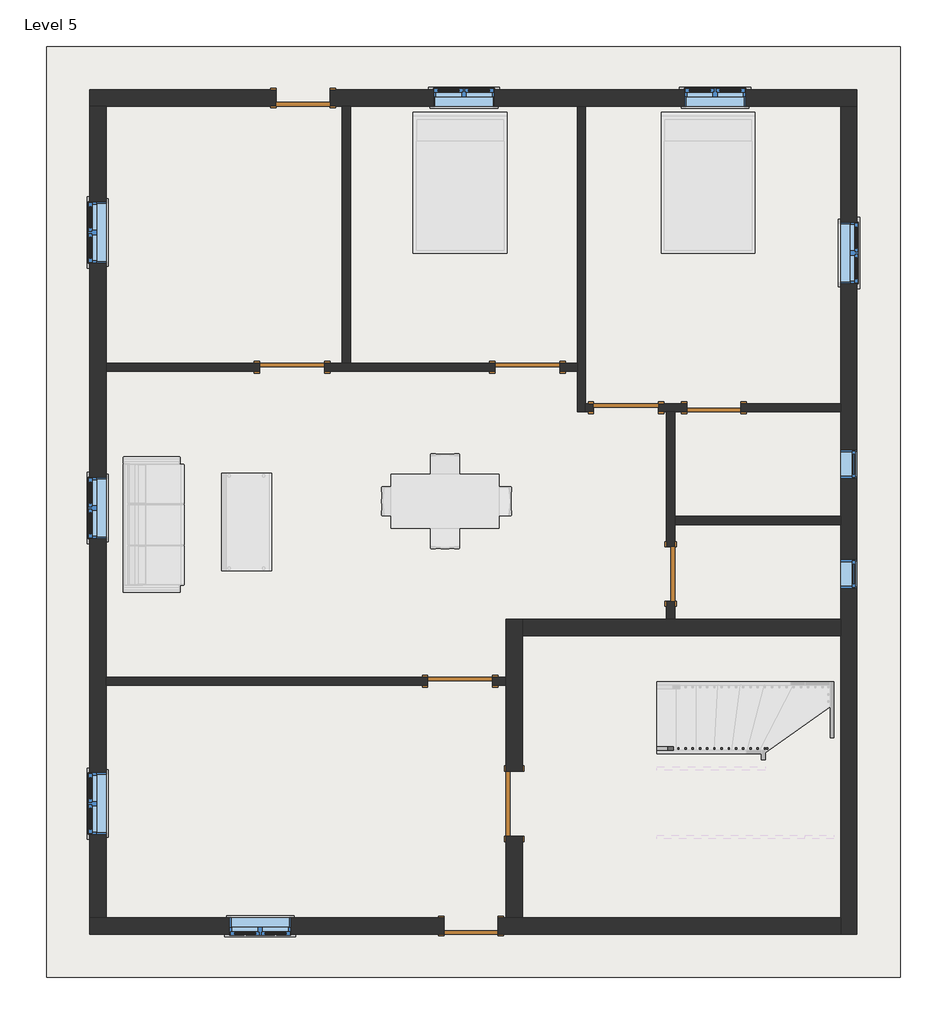
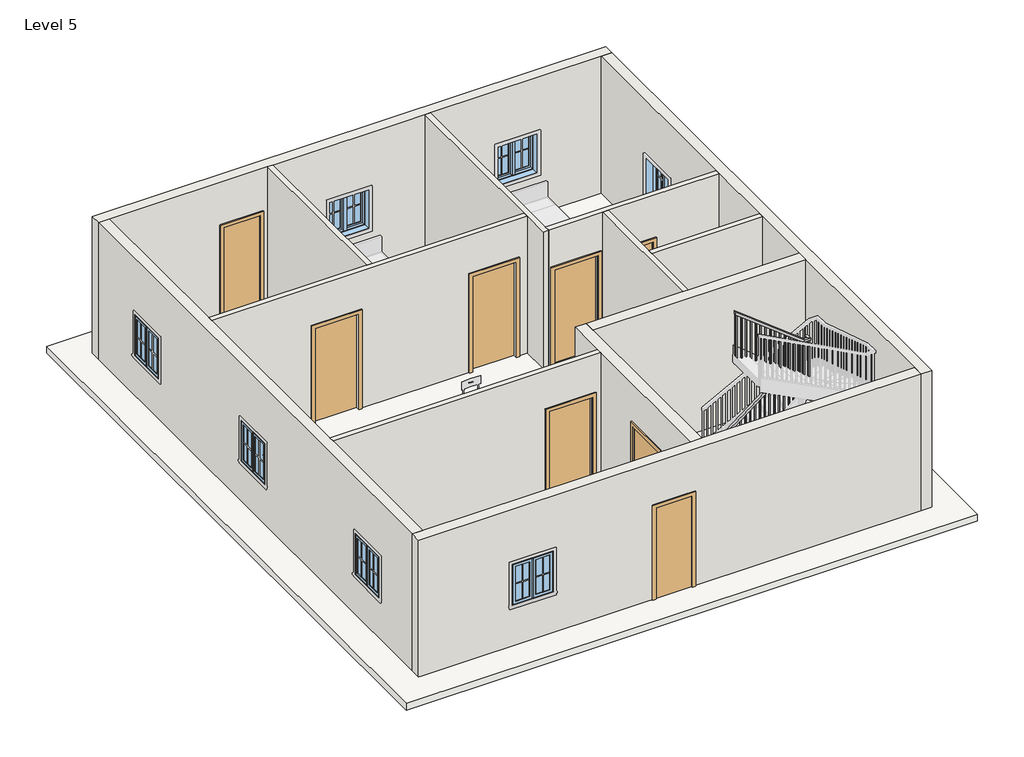
# One storey, part 1 of 2: 13 walls, 9 doors, 9 windows, 1 railing, 1 roof.
"""IFC4 building model written with IfcOpenShell, lengths in millimetres."""

from ifc_helpers import new_model, si_unit, frame, origin, place, context, project, spatial, polyline, outline, extrude, faceted_brep, transform, mapped, element, save
from components import door_85036156, door_d8f5dbb5, door_a1484949, door_e5f9f3c4, door_305aa2a5, door_0ca8825f, window_aa618e30, window_339605e1

model = new_model("IFC4")

# Units and contexts
model_context = context("Model", 3, world=origin())
ifc_project = project(units=[si_unit("LENGTHUNIT", "METRE", prefix="MILLI")], contexts=[model_context])

# Site, building, storey
site = spatial("IfcSite", under=ifc_project)
building = spatial("IfcBuilding", under=site)
storey = spatial("IfcBuildingStorey", under=building, Name="Level 5", Elevation=9601.2)

# Doors
placement = place(None, origin())
door_shape = door_85036156(model_context)
element("IfcDoor", 1, ObjectType="Single-Flush : 30\" x 80\"", at=placement, inside=storey, context=model_context, shape_type="MappedRepresentation", body=[
    mapped(door_shape, transform((-3639.3817864, 7024.9034997, 9601.2), x_axis=(1.0, 0.0, 0.0), y_axis=(0.0, 1.0, 0.0), z_axis=(0.0, 0.0, 1.0))),
])
door_2_shape = door_d8f5dbb5(model_context)
element("IfcDoor", 2, ObjectType="Single-Flush : 30\" x 80\"", at=placement, inside=storey, context=model_context, shape_type="MappedRepresentation", body=[
    mapped(door_2_shape, transform((2149.2782136, 2662.4534997, 9601.2), x_axis=(-1.0, 0.0, 0.0), y_axis=(0.0, -1.0, 0.0), z_axis=(0.0, 0.0, 1.0))),
])
element("IfcDoor", 3, ObjectType="Single-Flush : 30\" x 80\"", at=placement, inside=storey, context=model_context, shape_type="MappedRepresentation", body=[
    mapped(door_2_shape, transform((1539.6782136, 322.4784997, 9601.2), x_axis=(0.0, -1.0, 0.0), y_axis=(1.0, 0.0, 0.0), z_axis=(0.0, 0.0, 1.0))),
])
door_3_shape = door_a1484949(model_context)
element("IfcDoor", 4, ObjectType="Single-Flush : 30\" x 80\"", at=placement, inside=storey, context=model_context, shape_type="MappedRepresentation", body=[
    mapped(door_3_shape, transform((-1273.3717864, -4633.6965003, 9601.2), x_axis=(-1.0, 0.0, 0.0), y_axis=(0.0, -1.0, 0.0), z_axis=(0.0, 0.0, 1.0))),
])
door_4_shape = door_e5f9f3c4(model_context)
element("IfcDoor", 5, ObjectType="Single-Flush : 36\" x 84\"", at=placement, inside=storey, context=model_context, shape_type="MappedRepresentation", body=[
    mapped(door_4_shape, transform((-477.0817864, 3233.9534997, 9601.2), x_axis=(1.0, 0.0, 0.0), y_axis=(0.0, 1.0, 0.0), z_axis=(0.0, 0.0, 1.0))),
])
element("IfcDoor", 6, ObjectType="Single-Flush : 36\" x 84\"", at=placement, inside=storey, context=model_context, shape_type="MappedRepresentation", body=[
    mapped(door_4_shape, transform((-3791.7817864, 3233.9534997, 9601.2), x_axis=(1.0, 0.0, 0.0), y_axis=(0.0, 1.0, 0.0), z_axis=(0.0, 0.0, 1.0))),
])
element("IfcDoor", 7, ObjectType="Single-Flush : 36\" x 84\"", at=placement, inside=storey, context=model_context, shape_type="MappedRepresentation", body=[
    mapped(door_4_shape, transform((-1425.7717864, -1188.1865003, 9601.2), x_axis=(1.0, 0.0, 0.0), y_axis=(0.0, 1.0, 0.0), z_axis=(0.0, 0.0, 1.0))),
])
door_5_shape = door_305aa2a5(model_context)
element("IfcDoor", 8, ObjectType="Single-Flush : 36\" x 84\"", at=placement, inside=storey, context=model_context, shape_type="MappedRepresentation", body=[
    mapped(door_5_shape, transform((912.2982136, 2662.4534997, 9601.2), x_axis=(-1.0, 0.0, 0.0), y_axis=(0.0, -1.0, 0.0), z_axis=(0.0, 0.0, 1.0))),
])
door_6_shape = door_0ca8825f(model_context)
element("IfcDoor", 9, ObjectType="Single-Flush : 36\" x 84\"", at=placement, inside=storey, context=model_context, shape_type="MappedRepresentation", body=[
    mapped(door_6_shape, transform((-663.7717864, -2910.9415003, 9601.2), x_axis=(0.0, 1.0, 0.0), y_axis=(-1.0, 0.0, 0.0), z_axis=(0.0, 0.0, 1.0))),
])

# Railing
element("IfcRailing", 10, ObjectType="Handrail - Rectangular", at=placement, inside=storey, context=model_context, shape_type="SolidModel", body=[
    faceted_brep([(1342.8282136, -2108.9365003, 10684.9333333), (1342.8282136, -2108.9365003, 10620.6000346), (1342.8282136, -2159.7365003, 10620.6000346), (1342.8282136, -2159.7365003, 10684.9333333), (2794.3599055, -2108.9365003, 11812.8191036), (2845.1599055, -2108.9365003, 11787.9590024), (2845.1599055, -2159.7365003, 11787.9590024), (2794.3599055, -2159.7365003, 11812.8191036), (2794.3599055, -2108.9365003, 12015.8281882), (2845.1599055, -2108.9365003, 11965.0281882), (2845.1599055, -2159.7365003, 11965.0281882), (2794.3599055, -2159.7365003, 12015.8281882), (2921.3599055, -2108.9365003, 12015.8281882), (2921.3599055, -2108.9365003, 11965.0281882), (2870.5599055, -2159.7365003, 11965.0281882), (2870.5599055, -2159.7365003, 12015.8281882), (2921.3599055, -2235.9365003, 12015.8281882), (2921.3599055, -2265.0578342, 11965.0281882), (2870.5599055, -2265.0578342, 11965.0281882), (2870.5599055, -2235.9365003, 12015.8281882), (2921.3599055, -2362.9365003, 12232.7051451), (2921.3599055, -2413.7365003, 12218.9256424), (2870.5599055, -2413.7365003, 12218.9256424), (2870.5599055, -2362.9365003, 12232.7051451), (2921.3599055, -2362.9365003, 12435.7142297), (2921.3599055, -2413.7365003, 12384.9142297), (2870.5599055, -2413.7365003, 12384.9142297), (2870.5599055, -2362.9365003, 12435.7142297), (2921.3599055, -2489.9365003, 12435.7142297), (2921.3599055, -2489.9365003, 12384.9142297), (2870.5599055, -2439.1365003, 12384.9142297), (2870.5599055, -2439.1365003, 12435.7142297), (2794.3599055, -2489.9365003, 12435.7142297), (2776.9432376, -2489.9365003, 12384.9142297), (2776.9432376, -2439.1365003, 12384.9142297), (2794.3599055, -2439.1365003, 12435.7142297), (1342.8282136, -2489.9365003, 13563.6), (1342.8282136, -2439.1365003, 13563.6), (1342.8282136, -2439.1365003, 13499.2667013), (1342.8282136, -2489.9365003, 13499.2667013)], [[[0, 1, 2, 3]], [[1, 0, 4, 5]], [[2, 1, 5, 6]], [[3, 2, 6, 7]], [[0, 3, 7, 4]], [[5, 4, 8, 9]], [[6, 5, 9, 10]], [[7, 6, 10, 11]], [[4, 7, 11, 8]], [[9, 8, 12, 13]], [[10, 9, 13, 14]], [[11, 10, 14, 15]], [[8, 11, 15, 12]], [[13, 12, 16, 17]], [[14, 13, 17, 18]], [[15, 14, 18, 19]], [[12, 15, 19, 16]], [[17, 16, 20, 21]], [[18, 17, 21, 22]], [[19, 18, 22, 23]], [[16, 19, 23, 20]], [[21, 20, 24, 25]], [[22, 21, 25, 26]], [[23, 22, 26, 27]], [[20, 23, 27, 24]], [[25, 24, 28, 29]], [[26, 25, 29, 30]], [[27, 26, 30, 31]], [[24, 27, 31, 28]], [[29, 28, 32, 33]], [[30, 29, 33, 34]], [[31, 30, 34, 35]], [[28, 31, 35, 32]], [[36, 37, 38, 39]], [[33, 32, 36, 39]], [[34, 33, 39, 38]], [[35, 34, 38, 37]], [[32, 35, 37, 36]]]),
    extrude(outline(polyline([(13469.2292361, 1381.4849055), (13484.0316852, 1362.4349055), (12479.8666667, 1362.4349055), (12479.8666667, 1381.4849055), (13469.2292361, 1381.4849055)])), frame((0.0, -2474.0615003, 0.0), z_axis=(0.0, 1.0, 0.0), x_axis=(0.0, 0.0, 1.0)), (0.0, 0.0, 1.0), 19.05),
    extrude(outline(polyline([(13390.2828411, 1483.0849055), (13405.0852902, 1464.0349055), (12479.8666667, 1464.0349055), (12479.8666667, 1483.0849055), (13390.2828411, 1483.0849055)])), frame((0.0, -2474.0615003, 0.0), z_axis=(0.0, 1.0, 0.0), x_axis=(0.0, 0.0, 1.0)), (0.0, 0.0, 1.0), 19.05),
    extrude(outline(polyline([(13311.3364462, 1584.6849055), (13326.1388952, 1565.6349055), (12479.8666667, 1565.6349055), (12479.8666667, 1584.6849055), (13311.3364462, 1584.6849055)])), frame((0.0, -2474.0615003, 0.0), z_axis=(0.0, 1.0, 0.0), x_axis=(0.0, 0.0, 1.0)), (0.0, 0.0, 1.0), 19.05),
    extrude(outline(polyline([(13232.3900512, 1686.2849055), (13247.1925003, 1667.2349055), (12310.5333333, 1667.2349055), (12310.5333333, 1686.2849055), (13232.3900512, 1686.2849055)])), frame((0.0, -2474.0615003, 0.0), z_axis=(0.0, 1.0, 0.0), x_axis=(0.0, 0.0, 1.0)), (0.0, 0.0, 1.0), 19.05),
    extrude(outline(polyline([(13153.4436562, 1787.8849055), (13168.2461053, 1768.8349055), (12310.5333333, 1768.8349055), (12310.5333333, 1787.8849055), (13153.4436562, 1787.8849055)])), frame((0.0, -2474.0615003, 0.0), z_axis=(0.0, 1.0, 0.0), x_axis=(0.0, 0.0, 1.0)), (0.0, 0.0, 1.0), 19.05),
    extrude(outline(polyline([(13074.4972613, 1889.4849055), (13089.2997103, 1870.4349055), (12310.5333333, 1870.4349055), (12310.5333333, 1889.4849055), (13074.4972613, 1889.4849055)])), frame((0.0, -2474.0615003, 0.0), z_axis=(0.0, 1.0, 0.0), x_axis=(0.0, 0.0, 1.0)), (0.0, 0.0, 1.0), 19.05),
    extrude(outline(polyline([(12995.5508663, 1991.0849055), (13010.3533154, 1972.0349055), (12141.2, 1972.0349055), (12141.2, 1991.0849055), (12995.5508663, 1991.0849055)])), frame((0.0, -2474.0615003, 0.0), z_axis=(0.0, 1.0, 0.0), x_axis=(0.0, 0.0, 1.0)), (0.0, 0.0, 1.0), 19.05),
    extrude(outline(polyline([(12916.6044713, 2092.6849055), (12931.4069204, 2073.6349055), (12141.2, 2073.6349055), (12141.2, 2092.6849055), (12916.6044713, 2092.6849055)])), frame((0.0, -2474.0615003, 0.0), z_axis=(0.0, 1.0, 0.0), x_axis=(0.0, 0.0, 1.0)), (0.0, 0.0, 1.0), 19.05),
    extrude(outline(polyline([(12837.6580764, 2194.2849055), (12852.4605254, 2175.2349055), (11971.8666667, 2175.2349055), (11971.8666667, 2194.2849055), (12837.6580764, 2194.2849055)])), frame((0.0, -2474.0615003, 0.0), z_axis=(0.0, 1.0, 0.0), x_axis=(0.0, 0.0, 1.0)), (0.0, 0.0, 1.0), 19.05),
    extrude(outline(polyline([(12758.7116814, 2295.8849055), (12773.5141304, 2276.8349055), (11971.8666667, 2276.8349055), (11971.8666667, 2295.8849055), (12758.7116814, 2295.8849055)])), frame((0.0, -2474.0615003, 0.0), z_axis=(0.0, 1.0, 0.0), x_axis=(0.0, 0.0, 1.0)), (0.0, 0.0, 1.0), 19.05),
    extrude(outline(polyline([(12679.7652864, 2397.4849055), (12694.5677355, 2378.4349055), (11971.8666667, 2378.4349055), (11971.8666667, 2397.4849055), (12679.7652864, 2397.4849055)])), frame((0.0, -2474.0615003, 0.0), z_axis=(0.0, 1.0, 0.0), x_axis=(0.0, 0.0, 1.0)), (0.0, 0.0, 1.0), 19.05),
    extrude(outline(polyline([(12600.8188914, 2499.0849055), (12615.6213405, 2480.0349055), (11802.5333333, 2480.0349055), (11802.5333333, 2499.0849055), (12600.8188914, 2499.0849055)])), frame((0.0, -2474.0615003, 0.0), z_axis=(0.0, 1.0, 0.0), x_axis=(0.0, 0.0, 1.0)), (0.0, 0.0, 1.0), 19.05),
    extrude(outline(polyline([(12521.8724965, 2600.6849055), (12536.6749455, 2581.6349055), (11802.5333333, 2581.6349055), (11802.5333333, 2600.6849055), (12521.8724965, 2600.6849055)])), frame((0.0, -2474.0615003, 0.0), z_axis=(0.0, 1.0, 0.0), x_axis=(0.0, 0.0, 1.0)), (0.0, 0.0, 1.0), 19.05),
    extrude(outline(polyline([(12442.9261015, 2702.2849055), (12457.7285506, 2683.2349055), (11633.2, 2683.2349055), (11633.2, 2702.2849055), (12442.9261015, 2702.2849055)])), frame((0.0, -2474.0615003, 0.0), z_axis=(0.0, 1.0, 0.0), x_axis=(0.0, 0.0, 1.0)), (0.0, 0.0, 1.0), 19.05),
    extrude(outline(polyline([(12363.9797065, 2803.8849055), (12378.7821556, 2784.8349055), (11633.2, 2784.8349055), (11633.2, 2803.8849055), (12363.9797065, 2803.8849055)])), frame((0.0, -2474.0615003, 0.0), z_axis=(0.0, 1.0, 0.0), x_axis=(0.0, 0.0, 1.0)), (0.0, 0.0, 1.0), 19.05),
    extrude(outline(polyline([(2886.4349055, -2429.6115003), (2905.4849055, -2429.6115003), (2905.4849055, -2448.6615003), (2886.4349055, -2448.6615003), (2886.4349055, -2429.6115003)])), frame((0.0, 0.0, 11294.5333333), z_axis=(0.0, 0.0, 1.0), x_axis=(1.0, 0.0, 0.0)), (0.0, 0.0, 1.0), 1090.3808964),
    extrude(outline(polyline([(-2347.0615003, 12105.06524), (-2328.0115003, 12072.5336964), (-2328.0115003, 11125.2), (-2347.0615003, 11125.2), (-2347.0615003, 12105.06524)])), frame((2886.4349055, 0.0, 0.0), z_axis=(1.0, 0.0, 0.0), x_axis=(0.0, 1.0, 0.0)), (0.0, 0.0, 1.0), 19.05),
    extrude(outline(polyline([(-2245.4615003, 11931.5636744), (-2226.4115003, 11899.0321309), (-2226.4115003, 10955.8666667), (-2245.4615003, 10955.8666667), (-2245.4615003, 11931.5636744)])), frame((2886.4349055, 0.0, 0.0), z_axis=(1.0, 0.0, 0.0), x_axis=(0.0, 1.0, 0.0)), (0.0, 0.0, 1.0), 19.05),
    extrude(outline(polyline([(2857.3032136, -2143.8615003), (2857.3032136, -2124.8115003), (2876.3532136, -2124.8115003), (2876.3532136, -2143.8615003), (2857.3032136, -2143.8615003)])), frame((0.0, 0.0, 10786.5333333), z_axis=(0.0, 0.0, 1.0), x_axis=(1.0, 0.0, 0.0)), (0.0, 0.0, 1.0), 1178.4948549),
    extrude(outline(polyline([(11733.2507888, 2774.7532136), (11718.4483397, 2755.7032136), (10617.2, 2755.7032136), (10617.2, 2774.7532136), (11733.2507888, 2774.7532136)])), frame((0.0, -2143.8615003, 0.0), z_axis=(0.0, 1.0, 0.0), x_axis=(0.0, 0.0, 1.0)), (0.0, 0.0, 1.0), 19.05),
    extrude(outline(polyline([(11654.3043938, 2673.1532136), (11639.5019447, 2654.1032136), (10617.2, 2654.1032136), (10617.2, 2673.1532136), (11654.3043938, 2673.1532136)])), frame((0.0, -2143.8615003, 0.0), z_axis=(0.0, 1.0, 0.0), x_axis=(0.0, 0.0, 1.0)), (0.0, 0.0, 1.0), 19.05),
    extrude(outline(polyline([(11575.3579988, 2571.5532136), (11560.5555498, 2552.5032136), (10447.8666667, 2552.5032136), (10447.8666667, 2571.5532136), (11575.3579988, 2571.5532136)])), frame((0.0, -2143.8615003, 0.0), z_axis=(0.0, 1.0, 0.0), x_axis=(0.0, 0.0, 1.0)), (0.0, 0.0, 1.0), 19.05),
    extrude(outline(polyline([(11496.4116039, 2469.9532136), (11481.6091548, 2450.9032136), (10447.8666667, 2450.9032136), (10447.8666667, 2469.9532136), (11496.4116039, 2469.9532136)])), frame((0.0, -2143.8615003, 0.0), z_axis=(0.0, 1.0, 0.0), x_axis=(0.0, 0.0, 1.0)), (0.0, 0.0, 1.0), 19.05),
    extrude(outline(polyline([(11417.4652089, 2368.3532136), (11402.6627598, 2349.3032136), (10278.5333333, 2349.3032136), (10278.5333333, 2368.3532136), (11417.4652089, 2368.3532136)])), frame((0.0, -2143.8615003, 0.0), z_axis=(0.0, 1.0, 0.0), x_axis=(0.0, 0.0, 1.0)), (0.0, 0.0, 1.0), 19.05),
    extrude(outline(polyline([(11338.5188139, 2266.7532136), (11323.7163649, 2247.7032136), (10278.5333333, 2247.7032136), (10278.5333333, 2266.7532136), (11338.5188139, 2266.7532136)])), frame((0.0, -2143.8615003, 0.0), z_axis=(0.0, 1.0, 0.0), x_axis=(0.0, 0.0, 1.0)), (0.0, 0.0, 1.0), 19.05),
    extrude(outline(polyline([(11259.5724189, 2165.1532136), (11244.7699699, 2146.1032136), (10109.2, 2146.1032136), (10109.2, 2165.1532136), (11259.5724189, 2165.1532136)])), frame((0.0, -2143.8615003, 0.0), z_axis=(0.0, 1.0, 0.0), x_axis=(0.0, 0.0, 1.0)), (0.0, 0.0, 1.0), 19.05),
    extrude(outline(polyline([(11180.626024, 2063.5532136), (11165.8235749, 2044.5032136), (10109.2, 2044.5032136), (10109.2, 2063.5532136), (11180.626024, 2063.5532136)])), frame((0.0, -2143.8615003, 0.0), z_axis=(0.0, 1.0, 0.0), x_axis=(0.0, 0.0, 1.0)), (0.0, 0.0, 1.0), 19.05),
    extrude(outline(polyline([(11101.679629, 1961.9532136), (11086.8771799, 1942.9032136), (10109.2, 1942.9032136), (10109.2, 1961.9532136), (11101.679629, 1961.9532136)])), frame((0.0, -2143.8615003, 0.0), z_axis=(0.0, 1.0, 0.0), x_axis=(0.0, 0.0, 1.0)), (0.0, 0.0, 1.0), 19.05),
    extrude(outline(polyline([(11022.733234, 1860.3532136), (11007.930785, 1841.3032136), (9939.8666667, 1841.3032136), (9939.8666667, 1860.3532136), (11022.733234, 1860.3532136)])), frame((0.0, -2143.8615003, 0.0), z_axis=(0.0, 1.0, 0.0), x_axis=(0.0, 0.0, 1.0)), (0.0, 0.0, 1.0), 19.05),
    extrude(outline(polyline([(10943.7868391, 1758.7532136), (10928.98439, 1739.7032136), (9939.8666667, 1739.7032136), (9939.8666667, 1758.7532136), (10943.7868391, 1758.7532136)])), frame((0.0, -2143.8615003, 0.0), z_axis=(0.0, 1.0, 0.0), x_axis=(0.0, 0.0, 1.0)), (0.0, 0.0, 1.0), 19.05),
    extrude(outline(polyline([(10864.8404441, 1657.1532136), (10850.037995, 1638.1032136), (9939.8666667, 1638.1032136), (9939.8666667, 1657.1532136), (10864.8404441, 1657.1532136)])), frame((0.0, -2143.8615003, 0.0), z_axis=(0.0, 1.0, 0.0), x_axis=(0.0, 0.0, 1.0)), (0.0, 0.0, 1.0), 19.05),
    extrude(outline(polyline([(10785.8940491, 1555.5532136), (10771.0916001, 1536.5032136), (9770.5333333, 1536.5032136), (9770.5333333, 1555.5532136), (10785.8940491, 1555.5532136)])), frame((0.0, -2143.8615003, 0.0), z_axis=(0.0, 1.0, 0.0), x_axis=(0.0, 0.0, 1.0)), (0.0, 0.0, 1.0), 19.05),
    extrude(outline(polyline([(10706.9476541, 1453.9532136), (10692.1452051, 1434.9032136), (9770.5333333, 1434.9032136), (9770.5333333, 1453.9532136), (10706.9476541, 1453.9532136)])), frame((0.0, -2143.8615003, 0.0), z_axis=(0.0, 1.0, 0.0), x_axis=(0.0, 0.0, 1.0)), (0.0, 0.0, 1.0), 19.05),
    extrude(outline(polyline([(2886.4349055, -2455.0115003), (2905.4849055, -2455.0115003), (2905.4849055, -2474.0615003), (2886.4349055, -2474.0615003), (2886.4349055, -2455.0115003)])), frame((0.0, 0.0, 11463.8666667), z_axis=(0.0, 0.0, 1.0), x_axis=(1.0, 0.0, 0.0)), (0.0, 0.0, 1.0), 921.0475631),
    extrude(outline(polyline([(2886.4349055, -2143.8615003), (2886.4349055, -2124.8115003), (2905.4849055, -2124.8115003), (2905.4849055, -2143.8615003), (2886.4349055, -2143.8615003)])), frame((0.0, 0.0, 10786.5333333), z_axis=(0.0, 0.0, 1.0), x_axis=(1.0, 0.0, 0.0)), (0.0, 0.0, 1.0), 1178.4948549),
    extrude(outline(polyline([(13484.4642523, 1361.8782136), (13499.2667013, 1342.8282136), (12479.8666667, 1342.8282136), (12479.8666667, 1361.8782136), (13484.4642523, 1361.8782136)])), frame((0.0, -2474.0615003, 0.0), z_axis=(0.0, 1.0, 0.0), x_axis=(0.0, 0.0, 1.0)), (0.0, 0.0, 1.0), 19.05),
    extrude(outline(polyline([(10635.4024837, 1361.8782136), (10620.6000346, 1342.8282136), (9770.5333333, 1342.8282136), (9770.5333333, 1361.8782136), (10635.4024837, 1361.8782136)])), frame((0.0, -2143.8615003, 0.0), z_axis=(0.0, 1.0, 0.0), x_axis=(0.0, 0.0, 1.0)), (0.0, 0.0, 1.0), 19.05),
])

# Roof
element("IfcRoof", 11, ObjectType="Generic - 12\"", at=placement, inside=storey, context=model_context, shape_type="SweptSolid", body=[
    extrude(outline(polyline([(-7252.5317864, 7748.8034997), (4771.8282136, 7748.8034997), (4771.8282136, -5357.5965003), (-7252.5317864, -5357.5965003), (-7252.5317864, 7748.8034997)])), frame((0.0, 0.0, 9448.8), z_axis=(0.0, 0.0, 1.0), x_axis=(1.0, 0.0, 0.0)), (0.0, 0.0, 1.0), 152.4),
])

# Walls
element("IfcWall", 12, ObjectType="WALL4.5\"", at=placement, inside=storey, context=model_context, shape_type="Brep", body=[
    faceted_brep([(-3334.5817864, 3176.8034997, 11734.8), (-3334.5817864, 3176.8034997, 9601.2), (-934.2817864, 3176.8034997, 9601.2), (-934.2817864, 3176.8034997, 11734.8), (-19.8817864, 3176.8034997, 11734.8), (-19.8817864, 3176.8034997, 9601.2), (227.7682136, 3176.8034997, 9601.2), (227.7682136, 3176.8034997, 12649.2), (-6414.3317864, 3176.8034997, 12649.2), (-6414.3317864, 3176.8034997, 9601.2), (-4248.9817864, 3176.8034997, 9601.2), (-4248.9817864, 3176.8034997, 11734.8), (-934.2817864, 3291.1034997, 9601.2), (-2972.6317864, 3291.1034997, 9601.2), (-3086.9317864, 3291.1034997, 9601.2), (-3334.5817864, 3291.1034997, 9601.2), (-3334.5817864, 3291.1034997, 11734.8), (-4248.9817864, 3291.1034997, 11734.8), (-4248.9817864, 3291.1034997, 9601.2), (-6414.3317864, 3291.1034997, 9601.2), (-6414.3317864, 3291.1034997, 12649.2), (-3086.9317864, 3291.1034997, 12649.2), (-2972.6317864, 3291.1034997, 12649.2), (227.7682136, 3291.1034997, 12649.2), (227.7682136, 3291.1034997, 9601.2), (-19.8817864, 3291.1034997, 9601.2), (-19.8817864, 3291.1034997, 11734.8), (-934.2817864, 3291.1034997, 11734.8)], [[[0, 1, 2, 3, 4, 5, 6, 7, 8, 9, 10, 11]], [[12, 13, 14, 15, 16, 17, 18, 19, 20, 21, 22, 23, 24, 25, 26, 27]], [[6, 5, 25, 24]], [[10, 9, 19, 18]], [[2, 1, 15, 14, 13, 12]], [[9, 8, 20, 19]], [[7, 6, 24, 23]], [[26, 25, 5, 4]], [[27, 26, 4, 3]], [[12, 27, 3, 2]], [[16, 15, 1, 0]], [[17, 16, 0, 11]], [[18, 17, 11, 10]], [[8, 7, 23, 22, 21, 20]]]),
])
element("IfcWall", 13, ObjectType="WALL4.5\"", at=placement, inside=storey, context=model_context, shape_type="Brep", body=[
    faceted_brep([(227.7682136, 6910.6034997, 9601.2), (227.7682136, 3291.1034997, 9601.2), (227.7682136, 3176.8034997, 9601.2), (227.7682136, 2605.3034997, 9601.2), (227.7682136, 2605.3034997, 12649.2), (227.7682136, 3176.8034997, 12649.2), (227.7682136, 3291.1034997, 12649.2), (227.7682136, 6910.6034997, 12649.2), (342.0682136, 6910.6034997, 9601.2), (342.0682136, 6910.6034997, 12649.2), (342.0682136, 2719.6034997, 12649.2), (342.0682136, 2605.3034997, 12649.2), (342.0682136, 2605.3034997, 9601.2), (342.0682136, 2719.6034997, 9601.2)], [[[0, 1, 2, 3, 4, 5, 6, 7]], [[8, 9, 10, 11, 12, 13]], [[3, 2, 1, 0, 8, 13, 12]], [[0, 7, 9, 8]], [[4, 3, 12, 11]], [[7, 6, 5, 4, 11, 10, 9]]]),
])
element("IfcWall", 14, ObjectType="WALL4.5\"", at=placement, inside=storey, context=model_context, shape_type="Brep", body=[
    faceted_brep([(1369.4982136, 2605.3034997, 9601.2), (1482.5282136, 2605.3034997, 9601.2), (1596.8282136, 2605.3034997, 9601.2), (1768.2782136, 2605.3034997, 9601.2), (1768.2782136, 2605.3034997, 11633.2), (2530.2782136, 2605.3034997, 11633.2), (2530.2782136, 2605.3034997, 9601.2), (3933.6282136, 2605.3034997, 9601.2), (3933.6282136, 2605.3034997, 12649.2), (1596.8282136, 2605.3034997, 12649.2), (1482.5282136, 2605.3034997, 12649.2), (342.0682136, 2605.3034997, 12649.2), (342.0682136, 2605.3034997, 9601.2), (455.0982136, 2605.3034997, 9601.2), (455.0982136, 2605.3034997, 11734.8), (1369.4982136, 2605.3034997, 11734.8), (1768.2782136, 2719.6034997, 11633.2), (1768.2782136, 2719.6034997, 9601.2), (1369.4982136, 2719.6034997, 9601.2), (1369.4982136, 2719.6034997, 11734.8), (455.0982136, 2719.6034997, 11734.8), (455.0982136, 2719.6034997, 9601.2), (342.0682136, 2719.6034997, 9601.2), (342.0682136, 2719.6034997, 12649.2), (3933.6282136, 2719.6034997, 12649.2), (3933.6282136, 2719.6034997, 9601.2), (2530.2782136, 2719.6034997, 9601.2), (2530.2782136, 2719.6034997, 11633.2)], [[[0, 1, 2, 3, 4, 5, 6, 7, 8, 9, 10, 11, 12, 13, 14, 15]], [[16, 17, 18, 19, 20, 21, 22, 23, 24, 25, 26, 27]], [[22, 21, 13, 12]], [[26, 25, 7, 6]], [[18, 17, 3, 2, 1, 0]], [[12, 11, 23, 22]], [[8, 7, 25, 24]], [[14, 13, 21, 20]], [[15, 14, 20, 19]], [[0, 15, 19, 18]], [[4, 3, 17, 16]], [[5, 4, 16, 27]], [[6, 5, 27, 26]], [[11, 10, 9, 8, 24, 23]]]),
])
element("IfcWall", 15, ObjectType="WALL4.5\"", at=placement, inside=storey, context=model_context, shape_type="SweptSolid", body=[
    extrude(outline(polyline([(-3086.9317864, 3291.1034997), (-3086.9317864, 6910.6034997), (-2972.6317864, 6910.6034997), (-2972.6317864, 3291.1034997), (-3086.9317864, 3291.1034997)])), frame((0.0, 0.0, 9601.2), z_axis=(0.0, 0.0, 1.0), x_axis=(1.0, 0.0, 0.0)), (0.0, 0.0, 1.0), 3048.0),
])
element("IfcWall", 16, ObjectType="WALL4.5\"", at=placement, inside=storey, context=model_context, shape_type="Brep", body=[
    faceted_brep([(1482.5282136, -58.5215003, 11633.2), (1482.5282136, -58.5215003, 9601.2), (1482.5282136, -315.6965003, 9601.2), (1482.5282136, -315.6965003, 12649.2), (1482.5282136, 2605.3034997, 12649.2), (1482.5282136, 2605.3034997, 9601.2), (1482.5282136, 703.4784997, 9601.2), (1482.5282136, 703.4784997, 11633.2), (1596.8282136, -315.6965003, 9601.2), (1596.8282136, -58.5215003, 9601.2), (1596.8282136, -58.5215003, 11633.2), (1596.8282136, 703.4784997, 11633.2), (1596.8282136, 703.4784997, 9601.2), (1596.8282136, 1017.8034997, 9601.2), (1596.8282136, 1132.1034997, 9601.2), (1596.8282136, 2605.3034997, 9601.2), (1596.8282136, 2605.3034997, 12649.2), (1596.8282136, 1132.1034997, 12649.2), (1596.8282136, 1017.8034997, 12649.2), (1596.8282136, -315.6965003, 12649.2)], [[[0, 1, 2, 3, 4, 5, 6, 7]], [[8, 9, 10, 11, 12, 13, 14, 15, 16, 17, 18, 19]], [[6, 5, 15, 14, 13, 12]], [[2, 1, 9, 8]], [[5, 4, 16, 15]], [[3, 2, 8, 19]], [[10, 9, 1, 0]], [[11, 10, 0, 7]], [[12, 11, 7, 6]], [[4, 3, 19, 18, 17, 16]]]),
])
element("IfcWall", 17, ObjectType="WALL4.5\"", at=placement, inside=storey, context=model_context, shape_type="SweptSolid", body=[
    extrude(outline(polyline([(3933.6282136, 1017.8034997), (1596.8282136, 1017.8034997), (1596.8282136, 1132.1034997), (3933.6282136, 1132.1034997), (3933.6282136, 1017.8034997)])), frame((0.0, 0.0, 9601.2), z_axis=(0.0, 0.0, 1.0), x_axis=(1.0, 0.0, 0.0)), (0.0, 0.0, 1.0), 3048.0),
])
element("IfcWall", 18, ObjectType="WALL4.5\"", at=placement, inside=storey, context=model_context, shape_type="SweptSolid", body=[
    extrude(outline(polyline([(11734.8, -968.5717864), (9601.2, -968.5717864), (9601.2, -778.0717864), (12649.2, -778.0717864), (12649.2, -6414.3317864), (9601.2, -6414.3317864), (9601.2, -1882.9717864), (11734.8, -1882.9717864), (11734.8, -968.5717864)])), frame((0.0, -1245.3365003, 0.0), z_axis=(0.0, 1.0, 0.0), x_axis=(0.0, 0.0, 1.0)), (0.0, 0.0, 1.0), 114.3),
])
element("IfcWall", 19, ObjectType="WALL9\"", at=placement, inside=storey, context=model_context, shape_type="Brep", body=[
    faceted_brep([(-3258.3817864, 6910.6034997, 11633.2), (-3258.3817864, 6910.6034997, 9601.2), (-3086.9317864, 6910.6034997, 9601.2), (-2972.6317864, 6910.6034997, 9601.2), (227.7682136, 6910.6034997, 9601.2), (342.0682136, 6910.6034997, 9601.2), (3933.6282136, 6910.6034997, 9601.2), (4162.2282136, 6910.6034997, 9601.2), (4162.2282136, 6910.6034997, 12649.2), (3933.6282136, 6910.6034997, 12649.2), (342.0682136, 6910.6034997, 12649.2), (227.7682136, 6910.6034997, 12649.2), (-2972.6317864, 6910.6034997, 12649.2), (-3086.9317864, 6910.6034997, 12649.2), (-6414.3317864, 6910.6034997, 12649.2), (-6642.9317864, 6910.6034997, 12649.2), (-6642.9317864, 6910.6034997, 9601.2), (-6414.3317864, 6910.6034997, 9601.2), (-4020.3817864, 6910.6034997, 9601.2), (-4020.3817864, 6910.6034997, 11633.2), (-940.6317864, 6910.6034997, 11430.0), (-940.6317864, 6910.6034997, 10515.6), (-1804.2317864, 6910.6034997, 10515.6), (-1804.2317864, 6910.6034997, 11430.0), (2598.2232136, 6910.6034997, 11430.0), (2598.2232136, 6910.6034997, 10515.6), (1734.6232136, 6910.6034997, 10515.6), (1734.6232136, 6910.6034997, 11430.0), (4162.2282136, 7139.2034997, 9601.2), (-3258.3817864, 7139.2034997, 9601.2), (-3258.3817864, 7139.2034997, 11633.2), (-4020.3817864, 7139.2034997, 11633.2), (-4020.3817864, 7139.2034997, 9601.2), (-6642.9317864, 7139.2034997, 9601.2), (-6642.9317864, 7139.2034997, 12649.2), (4162.2282136, 7139.2034997, 12649.2), (-940.6317864, 7139.2034997, 11430.0), (-1804.2317864, 7139.2034997, 11430.0), (-1804.2317864, 7139.2034997, 10515.6), (-940.6317864, 7139.2034997, 10515.6), (2598.2232136, 7139.2034997, 11430.0), (1734.6232136, 7139.2034997, 11430.0), (1734.6232136, 7139.2034997, 10515.6), (2598.2232136, 7139.2034997, 10515.6)], [[[0, 1, 2, 3, 4, 5, 6, 7, 8, 9, 10, 11, 12, 13, 14, 15, 16, 17, 18, 19], [20, 21, 22, 23], [24, 25, 26, 27]], [[28, 29, 30, 31, 32, 33, 34, 35], [36, 37, 38, 39], [40, 41, 42, 43]], [[18, 17, 16, 33, 32]], [[7, 6, 5, 4, 3, 2, 1, 29, 28]], [[8, 7, 28, 35]], [[16, 15, 34, 33]], [[30, 29, 1, 0]], [[31, 30, 0, 19]], [[32, 31, 19, 18]], [[21, 20, 36, 39]], [[22, 21, 39, 38]], [[23, 22, 38, 37]], [[20, 23, 37, 36]], [[25, 24, 40, 43]], [[26, 25, 43, 42]], [[27, 26, 42, 41]], [[24, 27, 41, 40]], [[15, 14, 13, 12, 11, 10, 9, 8, 35, 34]]]),
])
element("IfcWall", 20, ObjectType="WALL9\"", at=placement, inside=storey, context=model_context, shape_type="Brep", body=[
    faceted_brep([(3933.6282136, 6910.6034997, 9601.2), (3933.6282136, 2719.6034997, 9601.2), (3933.6282136, 2605.3034997, 9601.2), (3933.6282136, 1132.1034997, 9601.2), (3933.6282136, 1017.8034997, 9601.2), (3933.6282136, -315.6965003, 9601.2), (3933.6282136, -544.2965003, 9601.2), (3933.6282136, -4519.3965003, 9601.2), (3933.6282136, -4747.9965003, 9601.2), (3933.6282136, -4747.9965003, 12649.2), (3933.6282136, -4519.3965003, 12649.2), (3933.6282136, -544.2965003, 12649.2), (3933.6282136, -315.6965003, 12649.2), (3933.6282136, 1017.8034997, 12649.2), (3933.6282136, 1132.1034997, 12649.2), (3933.6282136, 2605.3034997, 12649.2), (3933.6282136, 2719.6034997, 12649.2), (3933.6282136, 6910.6034997, 12649.2), (3933.6282136, 1665.5034997, 11125.2), (3933.6282136, 1665.5034997, 10515.6), (3933.6282136, 2071.9034997, 10515.6), (3933.6282136, 2071.9034997, 11125.2), (3933.6282136, 119.2784997, 11125.2), (3933.6282136, 119.2784997, 10515.6), (3933.6282136, 525.6784997, 10515.6), (3933.6282136, 525.6784997, 11125.2), (3933.6282136, 4411.8784997, 11430.0), (3933.6282136, 4411.8784997, 10515.6), (3933.6282136, 5275.4784997, 10515.6), (3933.6282136, 5275.4784997, 11430.0), (4162.2282136, 6910.6034997, 9601.2), (4162.2282136, 6910.6034997, 12649.2), (4162.2282136, -4747.9965003, 12649.2), (4162.2282136, -4747.9965003, 9601.2), (4162.2282136, 1665.5034997, 11125.2), (4162.2282136, 2071.9034997, 11125.2), (4162.2282136, 2071.9034997, 10515.6), (4162.2282136, 1665.5034997, 10515.6), (4162.2282136, 119.2784997, 11125.2), (4162.2282136, 525.6784997, 11125.2), (4162.2282136, 525.6784997, 10515.6), (4162.2282136, 119.2784997, 10515.6), (4162.2282136, 4411.8784997, 11430.0), (4162.2282136, 5275.4784997, 11430.0), (4162.2282136, 5275.4784997, 10515.6), (4162.2282136, 4411.8784997, 10515.6)], [[[0, 1, 2, 3, 4, 5, 6, 7, 8, 9, 10, 11, 12, 13, 14, 15, 16, 17], [18, 19, 20, 21], [22, 23, 24, 25], [26, 27, 28, 29]], [[30, 31, 32, 33], [34, 35, 36, 37], [38, 39, 40, 41], [42, 43, 44, 45]], [[8, 7, 6, 5, 4, 3, 2, 1, 0, 30, 33]], [[0, 17, 31, 30]], [[9, 8, 33, 32]], [[19, 18, 34, 37]], [[20, 19, 37, 36]], [[21, 20, 36, 35]], [[18, 21, 35, 34]], [[23, 22, 38, 41]], [[24, 23, 41, 40]], [[25, 24, 40, 39]], [[22, 25, 39, 38]], [[27, 26, 42, 45]], [[28, 27, 45, 44]], [[29, 28, 44, 43]], [[26, 29, 43, 42]], [[17, 16, 15, 14, 13, 12, 11, 10, 9, 32, 31]]]),
])
element("IfcWall", 21, ObjectType="WALL9\"", at=placement, inside=storey, context=model_context, shape_type="Brep", body=[
    faceted_brep([(-1654.3717864, -4519.3965003, 11633.2), (-1654.3717864, -4519.3965003, 9601.2), (-6414.3317864, -4519.3965003, 9601.2), (-6642.9317864, -4519.3965003, 9601.2), (-6642.9317864, -4519.3965003, 12649.2), (-6414.3317864, -4519.3965003, 12649.2), (-778.0717864, -4519.3965003, 12649.2), (-549.4717864, -4519.3965003, 12649.2), (3933.6282136, -4519.3965003, 12649.2), (3933.6282136, -4519.3965003, 9601.2), (-549.4717864, -4519.3965003, 9601.2), (-778.0717864, -4519.3965003, 9601.2), (-892.3717864, -4519.3965003, 9601.2), (-892.3717864, -4519.3965003, 11633.2), (-4674.4317864, -4519.3965003, 11430.0), (-4674.4317864, -4519.3965003, 10515.6), (-3810.8317864, -4519.3965003, 10515.6), (-3810.8317864, -4519.3965003, 11430.0), (-6642.9317864, -4747.9965003, 9601.2), (-1654.3717864, -4747.9965003, 9601.2), (-1654.3717864, -4747.9965003, 11633.2), (-892.3717864, -4747.9965003, 11633.2), (-892.3717864, -4747.9965003, 9601.2), (3933.6282136, -4747.9965003, 9601.2), (3933.6282136, -4747.9965003, 12649.2), (-6642.9317864, -4747.9965003, 12649.2), (-4674.4317864, -4747.9965003, 11430.0), (-3810.8317864, -4747.9965003, 11430.0), (-3810.8317864, -4747.9965003, 10515.6), (-4674.4317864, -4747.9965003, 10515.6)], [[[0, 1, 2, 3, 4, 5, 6, 7, 8, 9, 10, 11, 12, 13], [14, 15, 16, 17]], [[18, 19, 20, 21, 22, 23, 24, 25], [26, 27, 28, 29]], [[3, 2, 1, 19, 18]], [[12, 11, 10, 9, 23, 22]], [[9, 8, 24, 23]], [[4, 3, 18, 25]], [[15, 14, 26, 29]], [[16, 15, 29, 28]], [[17, 16, 28, 27]], [[14, 17, 27, 26]], [[8, 7, 6, 5, 4, 25, 24]], [[20, 19, 1, 0]], [[21, 20, 0, 13]], [[22, 21, 13, 12]]]),
])
element("IfcWall", 22, ObjectType="WALL9\"", at=placement, inside=storey, context=model_context, shape_type="Brep", body=[
    faceted_brep([(-6414.3317864, -4519.3965003, 9601.2), (-6414.3317864, -1245.3365003, 9601.2), (-6414.3317864, -1131.0365003, 9601.2), (-6414.3317864, 3176.8034997, 9601.2), (-6414.3317864, 3291.1034997, 9601.2), (-6414.3317864, 6910.6034997, 9601.2), (-6414.3317864, 6910.6034997, 12649.2), (-6414.3317864, 3291.1034997, 12649.2), (-6414.3317864, 3176.8034997, 12649.2), (-6414.3317864, -1131.0365003, 12649.2), (-6414.3317864, -1245.3365003, 12649.2), (-6414.3317864, -4519.3965003, 12649.2), (-6414.3317864, 5561.2284997, 11430.0), (-6414.3317864, 5561.2284997, 10515.6), (-6414.3317864, 4697.6284997, 10515.6), (-6414.3317864, 4697.6284997, 11430.0), (-6414.3317864, 1684.5534997, 11430.0), (-6414.3317864, 1684.5534997, 10515.6), (-6414.3317864, 820.9534997, 10515.6), (-6414.3317864, 820.9534997, 11430.0), (-6414.3317864, -2479.1415003, 11430.0), (-6414.3317864, -2479.1415003, 10515.6), (-6414.3317864, -3342.7415003, 10515.6), (-6414.3317864, -3342.7415003, 11430.0), (-6642.9317864, -4519.3965003, 9601.2), (-6642.9317864, -4519.3965003, 12649.2), (-6642.9317864, 6910.6034997, 12649.2), (-6642.9317864, 6910.6034997, 9601.2), (-6642.9317864, 5561.2284997, 11430.0), (-6642.9317864, 4697.6284997, 11430.0), (-6642.9317864, 4697.6284997, 10515.6), (-6642.9317864, 5561.2284997, 10515.6), (-6642.9317864, 1684.5534997, 11430.0), (-6642.9317864, 820.9534997, 11430.0), (-6642.9317864, 820.9534997, 10515.6), (-6642.9317864, 1684.5534997, 10515.6), (-6642.9317864, -2479.1415003, 11430.0), (-6642.9317864, -3342.7415003, 11430.0), (-6642.9317864, -3342.7415003, 10515.6), (-6642.9317864, -2479.1415003, 10515.6)], [[[0, 1, 2, 3, 4, 5, 6, 7, 8, 9, 10, 11], [12, 13, 14, 15], [16, 17, 18, 19], [20, 21, 22, 23]], [[24, 25, 26, 27], [28, 29, 30, 31], [32, 33, 34, 35], [36, 37, 38, 39]], [[5, 4, 3, 2, 1, 0, 24, 27]], [[0, 11, 25, 24]], [[6, 5, 27, 26]], [[13, 12, 28, 31]], [[14, 13, 31, 30]], [[15, 14, 30, 29]], [[12, 15, 29, 28]], [[17, 16, 32, 35]], [[18, 17, 35, 34]], [[19, 18, 34, 33]], [[16, 19, 33, 32]], [[21, 20, 36, 39]], [[22, 21, 39, 38]], [[23, 22, 38, 37]], [[20, 23, 37, 36]], [[11, 10, 9, 8, 7, 6, 26, 25]]]),
])
element("IfcWall", 23, ObjectType="WALL9\"", at=placement, inside=storey, context=model_context, shape_type="Brep", body=[
    faceted_brep([(-549.4717864, -2453.7415003, 11734.8), (-549.4717864, -2453.7415003, 9601.2), (-549.4717864, -544.2965003, 9601.2), (-549.4717864, -315.6965003, 9601.2), (-549.4717864, -315.6965003, 12649.2), (-549.4717864, -544.2965003, 12649.2), (-549.4717864, -4519.3965003, 12649.2), (-549.4717864, -4519.3965003, 9601.2), (-549.4717864, -3368.1415003, 9601.2), (-549.4717864, -3368.1415003, 11734.8), (-778.0717864, -315.6965003, 9601.2), (-778.0717864, -1131.0365003, 9601.2), (-778.0717864, -1245.3365003, 9601.2), (-778.0717864, -2453.7415003, 9601.2), (-778.0717864, -2453.7415003, 11734.8), (-778.0717864, -3368.1415003, 11734.8), (-778.0717864, -3368.1415003, 9601.2), (-778.0717864, -4519.3965003, 9601.2), (-778.0717864, -4519.3965003, 12649.2), (-778.0717864, -1245.3365003, 12649.2), (-778.0717864, -1131.0365003, 12649.2), (-778.0717864, -315.6965003, 12649.2)], [[[0, 1, 2, 3, 4, 5, 6, 7, 8, 9]], [[10, 11, 12, 13, 14, 15, 16, 17, 18, 19, 20, 21]], [[8, 7, 17, 16]], [[3, 2, 1, 13, 12, 11, 10]], [[7, 6, 18, 17]], [[4, 3, 10, 21]], [[14, 13, 1, 0]], [[15, 14, 0, 9]], [[16, 15, 9, 8]], [[6, 5, 4, 21, 20, 19, 18]]]),
])
element("IfcWall", 24, ObjectType="WALL9\"", at=placement, inside=storey, context=model_context, shape_type="Brep", body=[
    faceted_brep([(-549.4717864, -544.2965003, 9601.2), (3933.6282136, -544.2965003, 9601.2), (3933.6282136, -544.2965003, 12649.2), (-549.4717864, -544.2965003, 12649.2), (-549.4717864, -315.6965003, 9601.2), (-549.4717864, -315.6965003, 12649.2), (1482.5282136, -315.6965003, 12649.2), (1596.8282136, -315.6965003, 12649.2), (3933.6282136, -315.6965003, 12649.2), (3933.6282136, -315.6965003, 9601.2), (1596.8282136, -315.6965003, 9601.2), (1482.5282136, -315.6965003, 9601.2)], [[[0, 1, 2, 3]], [[4, 5, 6, 7, 8, 9, 10, 11]], [[1, 0, 4, 11, 10, 9]], [[0, 3, 5, 4]], [[2, 1, 9, 8]], [[3, 2, 8, 7, 6, 5]]]),
])

# Windows
window_shape = window_aa618e30(model_context)
element("IfcWindow", 25, ObjectType="Fixed : 16\" x 24\"", at=placement, inside=storey, context=model_context, shape_type="MappedRepresentation", body=[
    mapped(window_shape, transform((4047.9282136, 1830.6034997, 9601.2), x_axis=(0.0, -1.0, 0.0), y_axis=(1.0, 0.0, 0.0), z_axis=(0.0, 0.0, 1.0))),
])
element("IfcWindow", 26, ObjectType="Fixed : 16\" x 24\"", at=placement, inside=storey, context=model_context, shape_type="MappedRepresentation", body=[
    mapped(window_shape, transform((4047.9282136, 284.3784997, 9601.2), x_axis=(0.0, -1.0, 0.0), y_axis=(1.0, 0.0, 0.0), z_axis=(0.0, 0.0, 1.0))),
])
window_2_shape = window_339605e1(model_context)
element("IfcWindow", 27, ObjectType="Window-Casement-Double : 34\" x 36\"", at=placement, inside=storey, context=model_context, shape_type="MappedRepresentation", body=[
    mapped(window_2_shape, transform((-1372.4317864, 7024.9034997, 9601.2), x_axis=(1.0, 0.0, 0.0), y_axis=(0.0, 1.0, 0.0), z_axis=(0.0, 0.0, 1.0))),
])
element("IfcWindow", 28, ObjectType="Window-Casement-Double : 34\" x 36\"", at=placement, inside=storey, context=model_context, shape_type="MappedRepresentation", body=[
    mapped(window_2_shape, transform((2166.4232136, 7024.9034997, 9601.2), x_axis=(1.0, 0.0, 0.0), y_axis=(0.0, 1.0, 0.0), z_axis=(0.0, 0.0, 1.0))),
])
element("IfcWindow", 29, ObjectType="Window-Casement-Double : 34\" x 36\"", at=placement, inside=storey, context=model_context, shape_type="MappedRepresentation", body=[
    mapped(window_2_shape, transform((-6528.6317864, 5129.4284997, 9601.2), x_axis=(0.0, 1.0, 0.0), y_axis=(-1.0, 0.0, 0.0), z_axis=(0.0, 0.0, 1.0))),
])
element("IfcWindow", 30, ObjectType="Window-Casement-Double : 34\" x 36\"", at=placement, inside=storey, context=model_context, shape_type="MappedRepresentation", body=[
    mapped(window_2_shape, transform((-6528.6317864, 1252.7534997, 9601.2), x_axis=(0.0, 1.0, 0.0), y_axis=(-1.0, 0.0, 0.0), z_axis=(0.0, 0.0, 1.0))),
])
element("IfcWindow", 31, ObjectType="Window-Casement-Double : 34\" x 36\"", at=placement, inside=storey, context=model_context, shape_type="MappedRepresentation", body=[
    mapped(window_2_shape, transform((4047.9282136, 4843.6784997, 9601.2), x_axis=(0.0, -1.0, 0.0), y_axis=(1.0, 0.0, 0.0), z_axis=(0.0, 0.0, 1.0))),
])
element("IfcWindow", 32, ObjectType="Window-Casement-Double : 34\" x 36\"", at=placement, inside=storey, context=model_context, shape_type="MappedRepresentation", body=[
    mapped(window_2_shape, transform((-6528.6317864, -2910.9415003, 9601.2), x_axis=(0.0, 1.0, 0.0), y_axis=(-1.0, 0.0, 0.0), z_axis=(0.0, 0.0, 1.0))),
])
element("IfcWindow", 33, ObjectType="Window-Casement-Double : 34\" x 36\"", at=placement, inside=storey, context=model_context, shape_type="MappedRepresentation", body=[
    mapped(window_2_shape, transform((-4242.6317864, -4633.6965003, 9601.2), x_axis=(-1.0, 0.0, 0.0), y_axis=(0.0, -1.0, 0.0), z_axis=(0.0, 0.0, 1.0))),
])

save(model, "model.ifc")

# Revit data of these elements
# Type "Single-Flush : 30\" x 80\""
#   Type Mark = "5"
#   Construction Type Id = "MDOOR"
#   Assembly Code = "C1020"
#   Analytic Construction = "Metal"
#   Thickness = 0' - 2"
#   Heat Transfer Coefficient (U) = 0.651978 BTU/(h·ft²·°F)
#   Height = 6' - 8"
#   Trim Projection Ext = 0' - 1"
#   Trim Projection Int = 0' - 1"
#   Trim Width = 0' - 3"
#   Width = 2' - 6"
#   Define Thermal Properties by = 1
#   Define Thermal Properties by = 1
#   Door Material = Door - Panel
#   Frame Material = Door - Frame
#   Visual Light Transmittance = 0
#   Solar Heat Gain Coefficient = 0
#   Function = (empty or 0)
#   Wall Closure = (empty or 0)
# Type "Single-Flush : 36\" x 84\""
#   Type Mark = "1"
#   Construction Type Id = "MDOOR"
#   Assembly Code = "C1020"
#   Analytic Construction = "Metal"
#   Thickness = 0' - 2"
#   Heat Transfer Coefficient (U) = 0.651978 BTU/(h·ft²·°F)
#   Height = 7' - 0"
#   Trim Projection Ext = 0' - 1"
#   Trim Projection Int = 0' - 1"
#   Trim Width = 0' - 3"
#   Width = 3' - 0"
#   Define Thermal Properties by = 1
#   Define Thermal Properties by = 1
#   Door Material = Door - Panel
#   Frame Material = Door - Frame
#   Visual Light Transmittance = 0
#   Solar Heat Gain Coefficient = 0
#   Function = (empty or 0)
#   Wall Closure = (empty or 0)
# Type "Handrail - Rectangular"
#   Assembly Code = "C2010400"
#   built-in parameter 1008612 = 0.0416667 (stored number, unit not read)
#   built-in parameter 1008611 = 0.0416667 (stored number, unit not read)
#   built-in parameter 1008609 = 0.333333 (stored number, unit not read)
#   built-in parameter 1008604 = 0.166667 (stored number, unit not read)
#   built-in parameter 1008603 = 0.166667 (stored number, unit not read)
#   Railing Height = 3' - 0"
#   built-in parameter 1008630 = 2
#   built-in parameter 1008610 = 2
#   built-in parameter 1008618 = Baluster - Square : 3/4"
# Type "Generic - 12\""
#   Assembly Code = "B1020"
#   Layers, outside or top first: 0' - 6" no material (function 1)
# Type "WALL4.5\""
#   Assembly Code = "B2010"
#   Layers, outside or top first: 0' - 4 1/2" no material (function 1)
# Type "WALL9\""
#   Assembly Code = "B2010"
#   Layers, outside or top first: 0' - 9" no material (function 1)
# Type "Fixed : 16\" x 24\""
#   Type Mark = "4"
#   Construction Type Id = "GSP4R"
#   Assembly Code = "B2020100"
#   Analytic Construction = "1/8 in Pilkington single glazing"
#   Visual Light Transmittance = 0.9
#   Solar Heat Gain Coefficient = 0.78
#   Heat Transfer Coefficient (U) = 0.6496 BTU/(h·ft²·°F)
#   Height = 2' - 0"
#   Default Sill Height = 3' - 0"
#   Width = 1' - 4"
#   Window Inset = 0' - 0 3/4"
#   Define Thermal Properties by = 1
#   Define Thermal Properties by = 1
#   Glass Pane Material = Glass
#   Sash Material = Sash
#   Wall Closure = (empty or 0)
# Type "Window-Casement-Double : 34\" x 36\""
#   Type Mark = "14"
#   Fire Rating = "0.5h"
#   Assembly Code = "B2020100"
#   Analytic Construction = "Double glazing - domestic"
#   Frame Extension [instance default] = 0' - 0 1/4"
#   Window Inset [instance default] = 0' - 0"
#   Wall Thickness [instance default] = 0' - 6"
#   Interior Wall Closure [instance default] = 0' - 2 1/4"
#   Half Width = 1' - 5"
#   Visual Light Transmittance = 0.81
#   Thermal Resistance (R) = 1.8146 (h·ft²·°F)/BTU
#   Solar Heat Gain Coefficient = 0.76
#   Rough Width = 2' - 10 1/2"
#   Rough Height = 3' - 0 1/2"
#   Height = 3' - 0"
#   Heat Transfer Coefficient (U) = 0.5511 BTU/(h·ft²·°F)
#   Exterior Wall Closure [instance default] = 0' - 1 1/4"
#   Extension Jamb [instance default] = 0' - 2 1/4"
#   Default Sill Height = 3' - 0"
#   Width = 2' - 10"
#   Define Thermal Properties by = 0
#   Muntin Visibility = yes
#   Interior Trim Visibility [instance default] = yes
#   Exterior Trim Visibility [instance default] = yes
#   Extension Jamb Visibility [instance default] = yes
#   Interior Trim Material = Wood - Stained
#   Muntin Pattern = Muntin Pattern_2x2 : Muntin Pattern_2x2
#   Interior Trim = Trim-Window-Interior-Flat : Picture Frame
#   Interior Frame Material = Wood - Stained
#   Glass Panel Material = Glass
#   Exterior Trim Material = Clad - White
#   Exterior Trim = Trim-Window-Exterior-Flat : with Sill
#   Exterior Frame Material = Clad - White
#   Wall Closure = (empty or 0)
# Elements 1, 2, 3, 4 (IfcDoor, "Single-Flush : 30\" x 80\"")
#   Phase Created = New Construction
#   Materials on its faces: "Door - Frame", "Door - Panel"
# Elements 5, 6, 7, 8, 9 (IfcDoor, "Single-Flush : 36\" x 84\"")
#   Phase Created = New Construction
#   Materials on its faces: "Door - Frame", "Door - Panel"
# Element 10 (IfcRailing, "Handrail - Rectangular")
#   Phase Created = New Construction
# Element 11 (IfcRoof, "Generic - 12\"")
#   built-in parameter 1001705 = 31.5 (stored number, unit not read)
#   built-in parameter 1001701 = -0.5 (stored number, unit not read)
#   built-in parameter 1001710 = 33615
#   Phase Created = New Construction
#   Materials on its faces: "Default Roof"
# Elements 12, 13, 14, 15, 16, 17, 18 (IfcWall, "WALL4.5\"")
#   Top Offset = 0' - 0"
#   Base Offset = 0' - 0"
#   Unconnected Height = 10' - 0"
#   wall height = 10' - 0"
#   Phase Created = New Construction
#   Base Constraint = Level 5
#   Materials on its faces: "Default Wall"
# Elements 19, 20, 21, 22 (IfcWall, "WALL9\"")
#   Top Offset = 0' - 0"
#   Base Offset = 0' - 0"
#   Unconnected Height = 10' - 0"
#   wall height = 10' - 0"
#   Phase Created = New Construction
#   Base Constraint = Level 5
#   Materials on its faces: "Default Wall", "Wood Planks"
# Elements 23, 24 (IfcWall, "WALL9\"")
#   Top Offset = 0' - 0"
#   Base Offset = 0' - 0"
#   Unconnected Height = 10' - 0"
#   wall height = 10' - 0"
#   Phase Created = New Construction
#   Base Constraint = Level 5
#   Materials on its faces: "Default Wall"
# Element 25 (IfcWindow, "Fixed : 16\" x 24\"")
#   Mark = "28"
#   Phase Created = New Construction
#   Materials on its faces: "Sash", "Glass"
# Element 26 (IfcWindow, "Fixed : 16\" x 24\"")
#   Mark = "29"
#   Phase Created = New Construction
#   Materials on its faces: "Sash", "Glass"
# Element 27 (IfcWindow, "Window-Casement-Double : 34\" x 36\"")
#   Mark = "30"
#   Window Inset = 0' - 0"
#   Interior Wall Closure = 0' - 2 1/4"
#   Frame Extension = 0' - 0 1/4"
#   Exterior Wall Closure = 0' - 1 1/4"
#   Interior Trim Visibility = yes
#   Exterior Trim Visibility = yes
#   Phase Created = New Construction
#   Materials on its faces: "Wood - Stained", "Glass", "Clad - White"
# Element 28 (IfcWindow, "Window-Casement-Double : 34\" x 36\"")
#   Mark = "31"
#   Window Inset = 0' - 0"
#   Interior Wall Closure = 0' - 2 1/4"
#   Frame Extension = 0' - 0 1/4"
#   Exterior Wall Closure = 0' - 1 1/4"
#   Interior Trim Visibility = yes
#   Exterior Trim Visibility = yes
#   Phase Created = New Construction
#   Materials on its faces: "Wood - Stained", "Glass", "Clad - White"
# Element 29 (IfcWindow, "Window-Casement-Double : 34\" x 36\"")
#   Mark = "32"
#   Window Inset = 0' - 0"
#   Interior Wall Closure = 0' - 2 1/4"
#   Frame Extension = 0' - 0 1/4"
#   Exterior Wall Closure = 0' - 1 1/4"
#   Interior Trim Visibility = yes
#   Exterior Trim Visibility = yes
#   Phase Created = New Construction
#   Materials on its faces: "Wood - Stained", "Glass", "Clad - White"
# Element 30 (IfcWindow, "Window-Casement-Double : 34\" x 36\"")
#   Mark = "33"
#   Window Inset = 0' - 0"
#   Interior Wall Closure = 0' - 2 1/4"
#   Frame Extension = 0' - 0 1/4"
#   Exterior Wall Closure = 0' - 1 1/4"
#   Interior Trim Visibility = yes
#   Exterior Trim Visibility = yes
#   Phase Created = New Construction
#   Materials on its faces: "Wood - Stained", "Glass", "Clad - White"
# Element 31 (IfcWindow, "Window-Casement-Double : 34\" x 36\"")
#   Mark = "34"
#   Window Inset = 0' - 0"
#   Interior Wall Closure = 0' - 2 1/4"
#   Frame Extension = 0' - 0 1/4"
#   Exterior Wall Closure = 0' - 1 1/4"
#   Interior Trim Visibility = yes
#   Exterior Trim Visibility = yes
#   Phase Created = New Construction
#   Materials on its faces: "Wood - Stained", "Glass", "Clad - White"
# Element 32 (IfcWindow, "Window-Casement-Double : 34\" x 36\"")
#   Mark = "35"
#   Window Inset = 0' - 0"
#   Interior Wall Closure = 0' - 2 1/4"
#   Frame Extension = 0' - 0 1/4"
#   Exterior Wall Closure = 0' - 1 1/4"
#   Interior Trim Visibility = yes
#   Exterior Trim Visibility = yes
#   Phase Created = New Construction
#   Materials on its faces: "Wood - Stained", "Glass", "Clad - White"
# Element 33 (IfcWindow, "Window-Casement-Double : 34\" x 36\"")
#   Mark = "36"
#   Window Inset = 0' - 0"
#   Interior Wall Closure = 0' - 2 1/4"
#   Frame Extension = 0' - 0 1/4"
#   Exterior Wall Closure = 0' - 1 1/4"
#   Interior Trim Visibility = yes
#   Exterior Trim Visibility = yes
#   Phase Created = New Construction
#   Materials on its faces: "Wood - Stained", "Glass", "Clad - White"
# Materials
#   "Door - Panel": class "Wood", colour RGB 210 159 95, transparency 0, Cost = 0
#   "Door - Frame": colour RGB 118 70 51, transparency 0, Cost = 0
#   "Glass": class "Glass", colour RGB 0 128 192, transparency 0.75, Description = "Soda Lime Glass", Cost = 0
#   "Sash": class "Wood", colour RGB 224 178 126, transparency 0, Cost = 0
#   "Wood - Stained": class "Wood", colour RGB 224 178 126, transparency 0, Cost = 0
#   "Clad - White": class "Wood", colour RGB 242 242 238, transparency 0, Cost = 0
#   "Default Roof": colour RGB 88 101 114, transparency 0, Cost = 0
#   "Default Wall": colour RGB 128 128 128, transparency 0, Cost = 0
#   "Wood Planks": class "Wood", colour RGB 193 160 115, transparency 0, Description = "Physical material.", Cost = 0
